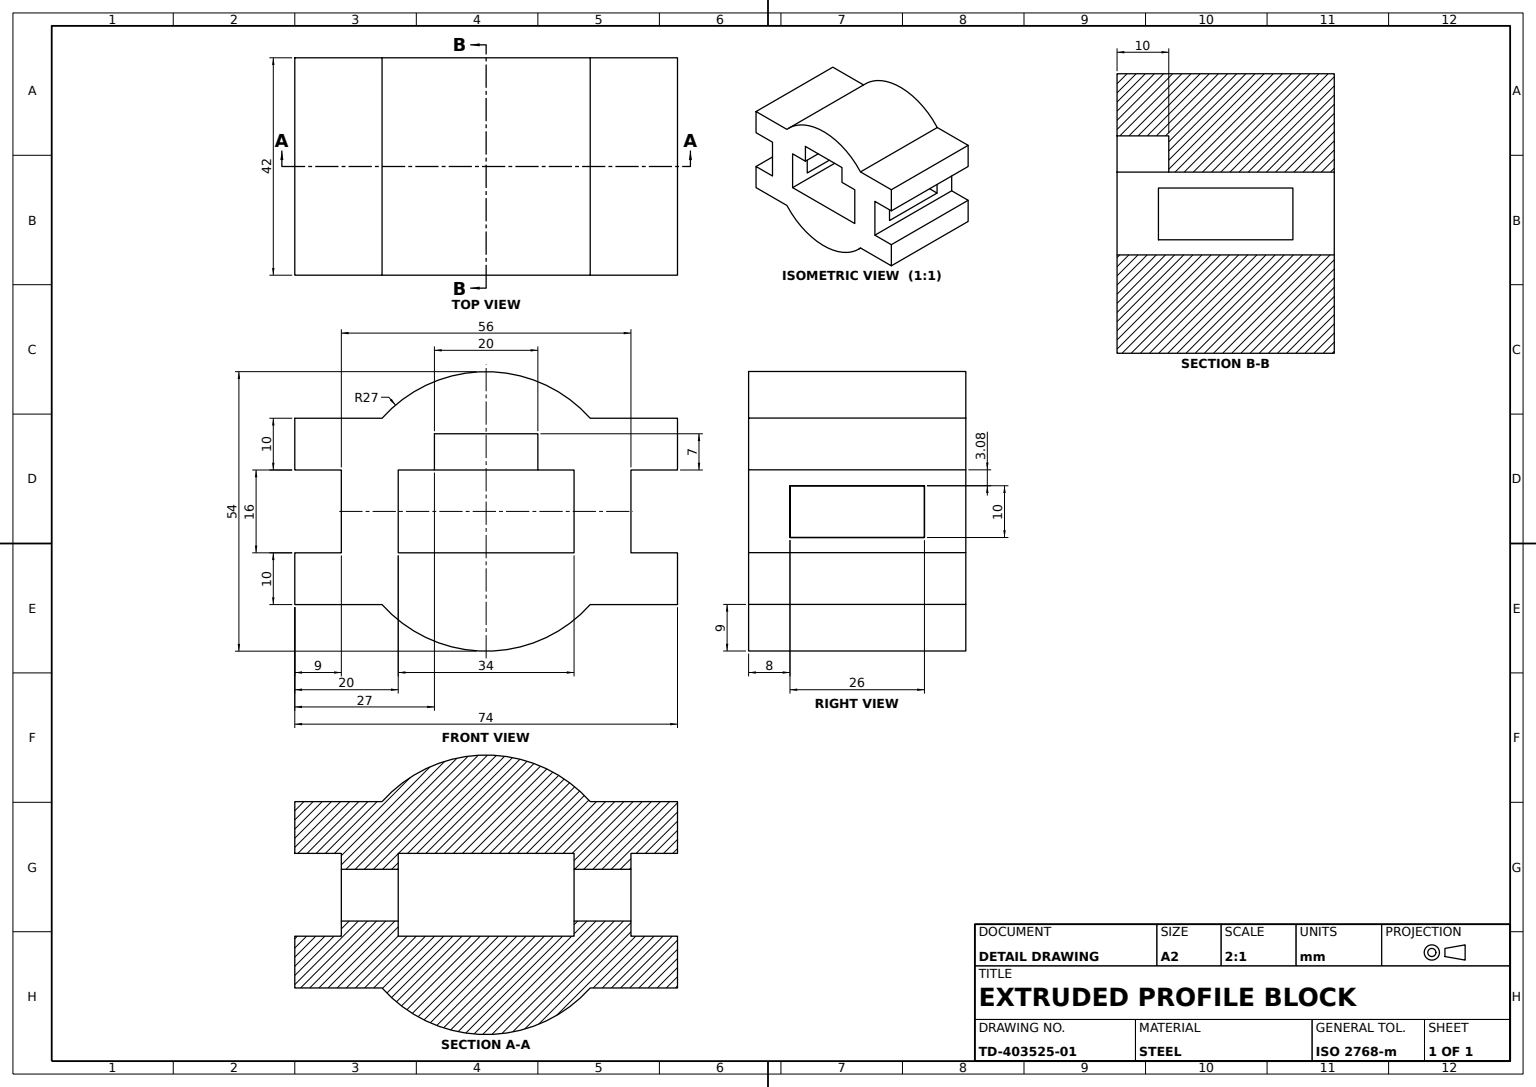
from build123d import *

# Parameters (mm, degrees)
BLOCK_EXTRUDE_42_DEPTH     = 42
THROUGH_WINDOW_CUT_DEPTH   = 97.254870007
POCKET_20X7_SKETCH_W       = 20
POCKET_20X7_SKETCH_H       = 7
POCKET_20X7_DEPTH_10_DEPTH = 10
SIDE_SLOT_SKETCH_W         = 26
SIDE_SLOT_SKETCH_H         = 10
SIDE_SLOT_CUT_26X8_DEPTH   = 90.520947269


with BuildPart() as part:
    # Block Profile Sketch → Block Extrude 42 (new body)
    with BuildSketch(Plane.XY):
        with BuildLine():
            Line((0, 0), (16.875388203, 0))
            ThreePointArc((16.875388203, 0), (37, 9), (57.124611797, 0))
            Line((57.124611797, 0), (74, 0))
            Line((74, 0), (74, -10))
            Line((74, -10), (65, -10))
            Line((65, -10), (65, -26))
            Line((65, -26), (74, -26))
            Line((74, -26), (74, -36))
            Line((74, -36), (57.124611797, -36))
            ThreePointArc((57.124611797, -36), (37, -45), (16.875388203, -36))
            Line((16.875388203, -36), (0, -36))
            Line((0, -36), (0, -26))
            Line((0, -26), (9, -26))
            Line((9, -26), (9, -10))
            Line((9, -10), (0, -10))
            Line((0, -10), (0, 0))
        make_face()
    extrude(amount=-BLOCK_EXTRUDE_42_DEPTH)

    # Through Window Sketch → Through Window Cut (cut, through all)
    with BuildSketch(Plane.XY):
        Polygon((47, -10), (54, -10), (54, -26), (20, -26), (20, -10), (27, -10), align=None)
    extrude(amount=-THROUGH_WINDOW_CUT_DEPTH, mode=Mode.SUBTRACT)

    # Pocket 20x7 Sketch → Pocket 20x7 Depth 10 (cut)
    with BuildSketch(Plane.XY):
        with Locations((37, -6.5)):
            Rectangle(POCKET_20X7_SKETCH_W, POCKET_20X7_SKETCH_H)
    extrude(amount=-POCKET_20X7_DEPTH_10_DEPTH, mode=Mode.SUBTRACT)

    # Side Slot Sketch → Side Slot Cut 26x8 (cut, through all)
    with BuildSketch(Plane.ZY.offset(-9)):
        with Locations((-21, -18.075177639)):
            Rectangle(SIDE_SLOT_SKETCH_W, SIDE_SLOT_SKETCH_H)
    extrude(amount=-SIDE_SLOT_CUT_26X8_DEPTH, mode=Mode.SUBTRACT)


solid = part.part
